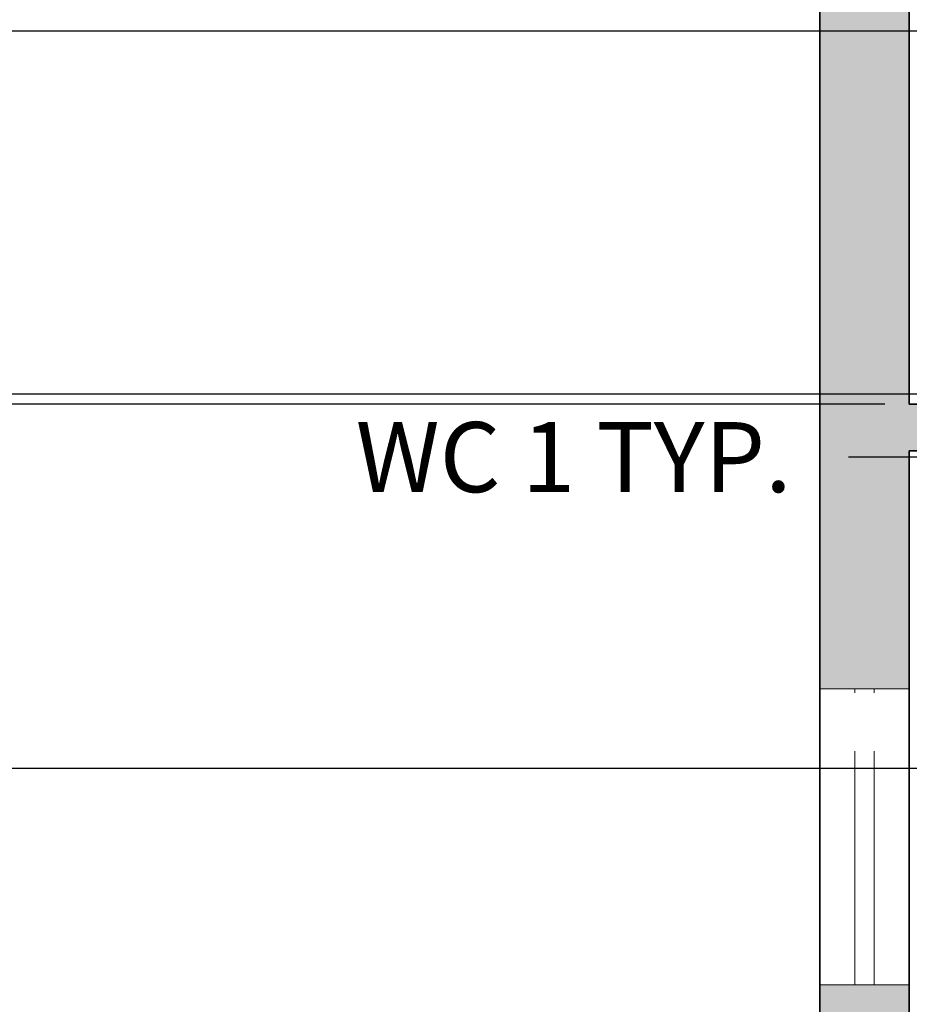
# Model space of a CAD drawing. Units: metres. Extents: x 4298.5 to 4325.2, y 2075 to 2095.8.
# Tile 12 of 35: x 4303.6 to 4305.9, y 2080.5 to 2083. Entities that reach past the tile are written whole.
import ezdxf

# ---------------------------------------------------------------- set-up
doc = ezdxf.new("R2010")
doc.units = ezdxf.units.M
doc.linetypes.add('ACAD_ISO02W100', pattern=[15, 12, -3])
for name, color, linetype, lineweight in [('A-ANNO-DIMS', 2, 'Continuous', 18), ('A-GLAZ', 4, 'Continuous', 18), ('A-GLAZ-OVHD', 4, 'ACAD_ISO02W100', 13), ('A-WALL', 7, 'Continuous', 35), ('A-WALL-PATT', 252, 'Continuous', 13)]:
    doc.layers.add(name, color=color, linetype=linetype, lineweight=lineweight)
doc.styles.get("Standard").update_dxf_attribs({"font": 'arial.ttf'})
doc.dimstyles.get("Standard").update_dxf_attribs({"dimtxt": 0.18, "dimasz": 0.18, "dimexe": 0.18, "dimexo": 0.0625, "dimgap": 0.09, "dimtad": 0, "dimtih": 1, "dimtoh": 1, "dimdec": 4, "dimzin": 0, "dimdsep": 46, "dimtxsty": 'Standard', "dimcen": 0.09, "dimadec": 0, "dimazin": 0, "dimtfac": 1, "dimtdec": 4, "dimtofl": 0, "dimtmove": 0, "dimatfit": 3, "dimfxl": 1, "dimtolj": 1, "dimtzin": 0, "dimarcsym": 0})

# ---------------------------------------------------------------- blocks, each defined once
blk = doc.blocks.new('WIN-760-GLASS-HIGH')
at = {"ltscale": 0.05}
for p, q in [((0, 0.76), (0, 0)), ((0.05, 0.76), (0.05, 0))]:
    blk.add_line(p, q, dxfattribs=at)
blk = doc.blocks.new('*D31')
at = {"layer": 'A-ANNO-DIMS', "color": 0, "lineweight": -2, "transparency": 16777216}
for p, q in [((4305.9147, 2081.8585), (4305.9147, 2082.1019)), ((4306.7541, 2081.8585), (4306.7541, 2082.1019)), ((4305.9147, 2081.9219), (4305.7347, 2081.9219)), ((4306.5741, 2081.9219), (4306.0947, 2081.9219))]:
    blk.add_line(p, q, dxfattribs=at)
at = {"layer": 'A-ANNO-DIMS', "color": 0, "transparency": 16777216}
for points in [[(4306.0947, 2081.9519), (4306.0947, 2081.8919), (4305.9147, 2081.9219)], [(4306.5741, 2081.9519), (4306.5741, 2081.8919), (4306.7541, 2081.9219)]]:
    blk.add_solid(points, dxfattribs=at)
at = {"layer": 'Defpoints', "color": 0, "transparency": 16777216}
for p in [(4305.9147, 2081.9219), (4305.9147, 2081.796), (4306.7541, 2081.796)]:
    blk.add_point(p, dxfattribs=at)
at = {"layer": 'A-ANNO-DIMS', "color": 0, "transparency": 16777216, "insert": (4305.0285, 2081.9219), "char_height": 0.18, "attachment_point": 5}
blk.add_mtext('\\A1;WC 1 TYP.', dxfattribs=at)
blk = doc.blocks.new('*D47')
at = {"layer": 'A-ANNO-DIMS', "color": 0, "lineweight": -2, "transparency": 16777216}
for p, q in [((4300.4306, 2084.4956), (4300.4306, 2074.9896)), ((4322.8106, 2084.4956), (4322.8106, 2074.9896)), ((4300.6106, 2075.1696), (4311.2252, 2075.1696)), ((4322.6306, 2075.1696), (4312.016, 2075.1696))]:
    blk.add_line(p, q, dxfattribs=at)
at = {"layer": 'A-ANNO-DIMS', "color": 0, "transparency": 16777216}
for points in [[(4300.6106, 2075.1996), (4300.6106, 2075.1396), (4300.4306, 2075.1696)], [(4322.6306, 2075.1996), (4322.6306, 2075.1396), (4322.8106, 2075.1696)]]:
    blk.add_solid(points, dxfattribs=at)
at = {"layer": 'Defpoints', "color": 0, "transparency": 16777216}
for p in [(4300.4306, 2084.5581), (4322.8106, 2084.5581), (4322.8106, 2075.1696)]:
    blk.add_point(p, dxfattribs=at)
at = {"layer": 'A-ANNO-DIMS', "color": 0, "transparency": 16777216, "insert": (4311.6206, 2075.1696), "char_height": 0.18, "attachment_point": 5}
blk.add_mtext('\\A1;22.38', dxfattribs=at)
blk = doc.blocks.new('*D51')
at = {"layer": 'A-ANNO-DIMS', "color": 0, "lineweight": -2, "transparency": 16777216}
for p, q in [((4305.5981, 2084.5581), (4299.0921, 2084.5581)), ((4299.2721, 2084.3781), (4299.2721, 2082.375)), ((4299.2721, 2080.0081), (4299.2721, 2082.0111)), ((4305.5981, 2079.8281), (4299.0921, 2079.8281))]:
    blk.add_line(p, q, dxfattribs=at)
at = {"layer": 'A-ANNO-DIMS', "color": 0, "transparency": 16777216}
for points in [[(4299.2421, 2084.3781), (4299.3021, 2084.3781), (4299.2721, 2084.5581)], [(4299.2421, 2080.0081), (4299.3021, 2080.0081), (4299.2721, 2079.8281)]]:
    blk.add_solid(points, dxfattribs=at)
at = {"layer": 'Defpoints', "color": 0, "transparency": 16777216}
for p in [(4305.6606, 2084.5581), (4299.2721, 2079.8281), (4305.6606, 2079.8281)]:
    blk.add_point(p, dxfattribs=at)
at = {"layer": 'A-ANNO-DIMS', "color": 0, "transparency": 16777216, "insert": (4299.2721, 2082.1931), "char_height": 0.18, "attachment_point": 5}
blk.add_mtext('\\A1;4.73', dxfattribs=at)
blk = doc.blocks.new('*D56')
at = {"layer": 'A-ANNO-DIMS', "color": 0, "lineweight": -2, "transparency": 16777216}
for p, q in [((4305.8281, 2085.0581), (4299.0921, 2085.0581)), ((4299.2721, 2084.8781), (4299.2721, 2083.74)), ((4299.2721, 2082.2381), (4299.2721, 2083.3761)), ((4305.8281, 2082.0581), (4299.0921, 2082.0581))]:
    blk.add_line(p, q, dxfattribs=at)
at = {"layer": 'A-ANNO-DIMS', "color": 0, "transparency": 16777216}
for points in [[(4299.2421, 2084.8781), (4299.3021, 2084.8781), (4299.2721, 2085.0581)], [(4299.2421, 2082.2381), (4299.3021, 2082.2381), (4299.2721, 2082.0581)]]:
    blk.add_solid(points, dxfattribs=at)
at = {"layer": 'Defpoints', "color": 0, "transparency": 16777216}
for p in [(4299.2721, 2085.0581), (4305.8906, 2085.0581), (4305.8906, 2082.0581)]:
    blk.add_point(p, dxfattribs=at)
at = {"layer": 'A-ANNO-DIMS', "color": 0, "transparency": 16777216, "insert": (4299.2721, 2083.5581), "char_height": 0.18, "attachment_point": 5}
blk.add_mtext('\\A1;3', dxfattribs=at)
blk = doc.blocks.new('*D62')
at = {"layer": 'A-ANNO-DIMS', "color": 0, "lineweight": -2, "transparency": 16777216}
for p, q in [((4312.1097, 2083.0153), (4299.0921, 2083.0153)), ((4299.2721, 2082.8353), (4299.2721, 2082.7313)), ((4299.2721, 2082.2635), (4299.2721, 2082.3674)), ((4312.1097, 2082.0835), (4299.0921, 2082.0835))]:
    blk.add_line(p, q, dxfattribs=at)
at = {"layer": 'A-ANNO-DIMS', "color": 0, "transparency": 16777216}
for points in [[(4299.2421, 2082.8353), (4299.3021, 2082.8353), (4299.2721, 2083.0153)], [(4299.2421, 2082.2635), (4299.3021, 2082.2635), (4299.2721, 2082.0835)]]:
    blk.add_solid(points, dxfattribs=at)
at = {"layer": 'Defpoints', "color": 0, "transparency": 16777216}
for p in [(4312.1722, 2083.0153), (4299.2721, 2082.0835), (4312.1722, 2082.0835)]:
    blk.add_point(p, dxfattribs=at)
at = {"layer": 'A-ANNO-DIMS', "color": 0, "transparency": 16777216, "insert": (4299.2721, 2082.5494), "char_height": 0.18, "attachment_point": 5}
blk.add_mtext('\\A1;0.93', dxfattribs=at)
blk = doc.blocks.new('*D63')
at = {"layer": 'A-ANNO-DIMS', "color": 0, "lineweight": -2, "transparency": 16777216}
for p, q in [((4312.1097, 2082.0835), (4299.0921, 2082.0835)), ((4299.2721, 2081.9035), (4299.2721, 2081.7847)), ((4299.2721, 2081.3021), (4299.2721, 2081.4209)), ((4312.1097, 2081.1221), (4299.0921, 2081.1221))]:
    blk.add_line(p, q, dxfattribs=at)
at = {"layer": 'A-ANNO-DIMS', "color": 0, "transparency": 16777216}
for points in [[(4299.2421, 2081.9035), (4299.3021, 2081.9035), (4299.2721, 2082.0835)], [(4299.2421, 2081.3021), (4299.3021, 2081.3021), (4299.2721, 2081.1221)]]:
    blk.add_solid(points, dxfattribs=at)
at = {"layer": 'Defpoints', "color": 0, "transparency": 16777216}
for p in [(4312.1722, 2082.0835), (4299.2721, 2081.1221), (4312.1722, 2081.1221)]:
    blk.add_point(p, dxfattribs=at)
at = {"layer": 'A-ANNO-DIMS', "color": 0, "transparency": 16777216, "insert": (4299.2721, 2081.6028), "char_height": 0.18, "attachment_point": 5}
blk.add_mtext('\\A1;0.96', dxfattribs=at)
blk = doc.blocks.new('*D64')
at = {"layer": 'A-ANNO-DIMS', "color": 0, "lineweight": -2, "transparency": 16777216}
for p, q in [((4312.1097, 2081.1221), (4299.0921, 2081.1221)), ((4299.2721, 2080.9421), (4299.2721, 2080.427)), ((4312.1097, 2080.247), (4299.0921, 2080.247)), ((4299.2721, 2080.247), (4299.2721, 2080.067)), ((4299.2721, 2080.067), (4299.0921, 2080.067))]:
    blk.add_line(p, q, dxfattribs=at)
at = {"layer": 'A-ANNO-DIMS', "color": 0, "transparency": 16777216}
for points in [[(4299.2421, 2080.9421), (4299.3021, 2080.9421), (4299.2721, 2081.1221)], [(4299.2421, 2080.427), (4299.3021, 2080.427), (4299.2721, 2080.247)]]:
    blk.add_solid(points, dxfattribs=at)
at = {"layer": 'Defpoints', "color": 0, "transparency": 16777216}
for p in [(4312.1722, 2081.1221), (4299.2721, 2080.247), (4312.1722, 2080.247)]:
    blk.add_point(p, dxfattribs=at)
at = {"layer": 'A-ANNO-DIMS', "color": 0, "transparency": 16777216, "insert": (4298.7681, 2080.067), "char_height": 0.18, "attachment_point": 5}
blk.add_mtext('\\A1;0.88', dxfattribs=at)

msp = doc.modelspace()

# ---------------------------------------------------------------- hatches: boundary and pattern name
at = {"layer": 'A-WALL-PATT'}
h = msp.add_hatch(color=256, dxfattribs=at)
h.dxf.hatch_style = 1
h.paths.add_polyline_path([(4308.7606, 2094.4781), (4308.1606, 2094.4781), (4307.4606, 2094.4781), (4307.4606, 2094.2481), (4308.2706, 2094.2481), (4308.2706, 2094.1281), (4308.3906, 2094.1281), (4308.3906, 2094.2481), (4308.7606, 2094.2481)])
h.paths.add_polyline_path([(4310.1206, 2094.4781), (4309.5206, 2094.4781), (4309.5206, 2094.2481), (4309.8906, 2094.2481), (4309.8906, 2092.2481), (4308.3906, 2092.2481), (4308.3906, 2093.4281), (4308.2706, 2093.4281), (4308.2706, 2092.0181), (4309.8906, 2092.0181), (4309.8906, 2087.0181), (4309.7706, 2087.0181), (4309.7706, 2086.7881), (4309.8906, 2086.7881), (4311.9406, 2086.7881), (4311.9406, 2087.0181), (4310.1206, 2087.0181), (4310.1206, 2089.0181), (4310.2406, 2089.0181), (4310.2406, 2089.1381), (4310.1206, 2089.1381), (4310.1206, 2092.0181), (4310.3078, 2092.0181), (4310.3078, 2092.2481), (4310.1206, 2092.2481)])
h.paths.add_polyline_path([(4311.7406, 2092.2481), (4311.0678, 2092.2481), (4311.0678, 2092.0181), (4311.7406, 2092.0181)], flags=17)
h.paths.add_polyline_path([(4313.1733, 2092.2481), (4312.5006, 2092.2481), (4312.5006, 2092.0181), (4313.1733, 2092.0181)])
h.paths.add_polyline_path([(4314.5378, 2092.2481), (4314.1206, 2092.2481), (4313.9333, 2092.2481), (4313.9333, 2092.0181), (4314.1206, 2092.0181), (4314.1206, 2087.0181), (4314.0006, 2087.0181), (4314.0006, 2086.7881), (4314.1206, 2086.7881), (4315.5718, 2086.7881), (4315.5718, 2087.0181), (4314.3506, 2087.0181), (4314.3506, 2092.0181), (4314.5378, 2092.0181)])
h.paths.add_polyline_path([(4315.9706, 2092.2481), (4315.2978, 2092.2481), (4315.2978, 2092.0181), (4315.9706, 2092.0181)])
h.paths.add_polyline_path([(4317.4033, 2092.2481), (4316.7306, 2092.2481), (4316.7306, 2092.0181), (4317.4033, 2092.0181)])
h.paths.add_polyline_path([(4318.9506, 2092.2481), (4318.3506, 2092.2481), (4318.1633, 2092.2481), (4318.1633, 2092.0181), (4318.3506, 2092.0181), (4318.3506, 2091.8981), (4318.5806, 2091.8981), (4318.5806, 2092.0181), (4318.9506, 2092.0181)])
h.paths.add_polyline_path([(4321.0106, 2092.2481), (4319.7106, 2092.2481), (4319.7106, 2092.0181), (4320.0806, 2092.0181), (4320.0806, 2090.0181), (4318.5806, 2090.0181), (4318.5806, 2091.1981), (4318.3506, 2091.1981), (4318.3506, 2090.0181), (4318.3506, 2087.0181), (4318.2306, 2087.0181), (4318.2306, 2086.7881), (4318.3506, 2086.7881), (4318.3506, 2086.3081), (4318.5806, 2086.3081), (4318.5806, 2089.7881), (4321.7806, 2089.7881), (4321.7806, 2090.0181), (4320.2006, 2090.0181), (4320.2006, 2092.0181), (4321.0106, 2092.0181)])
h.paths.add_polyline_path([(4322.8106, 2092.2481), (4321.7706, 2092.2481), (4321.7706, 2092.0181), (4322.5806, 2092.0181), (4322.5806, 2091.2831), (4322.8106, 2091.2831)])
h.paths.add_polyline_path([(4322.8106, 2090.5231), (4322.5806, 2090.5231), (4322.5806, 2089.7881), (4322.5806, 2089.5254), (4322.8106, 2089.5254), (4322.8106, 2090.0181)])
h.paths.add_polyline_path([(4322.8106, 2088.7654), (4322.5806, 2088.7654), (4322.5806, 2087.6681), (4322.8106, 2087.6681)])
h.paths.add_polyline_path([(4322.8106, 2086.9081), (4322.5806, 2086.9081), (4322.5806, 2085.8107), (4322.8106, 2085.8107)])
h.paths.add_polyline_path([(4322.8106, 2085.0507), (4322.5806, 2085.0507), (4322.5806, 2084.7881), (4318.5806, 2084.7881), (4318.5806, 2085.0581), (4318.5806, 2085.4081), (4318.3506, 2085.4081), (4318.3506, 2084.5581), (4318.3506, 2080.8581), (4318.4706, 2080.8581), (4318.4706, 2082.3281), (4319.2606, 2082.3281), (4319.2606, 2082.5581), (4318.5806, 2082.5581), (4318.5806, 2084.5581), (4320.0806, 2084.5581), (4320.0806, 2083.9381), (4320.3106, 2083.9381), (4320.3106, 2084.5581), (4322.8106, 2084.5581)])
h.paths.add_polyline_path([(4320.3106, 2083.1781), (4320.0806, 2083.1781), (4320.0806, 2082.5581), (4319.9606, 2082.5581), (4319.9606, 2082.3281), (4320.0806, 2082.3281), (4320.0806, 2081.5731), (4320.3106, 2081.5731)], flags=17)
h.paths.add_polyline_path([(4320.3106, 2080.8131), (4320.0806, 2080.8131), (4320.0806, 2080.0581), (4318.4286, 2080.0581), (4318.4286, 2079.8281), (4320.3106, 2079.8281)])
h.paths.add_polyline_path([(4317.3506, 2085.2881), (4316.5718, 2085.2881), (4316.5718, 2085.0581), (4317.3506, 2085.0581)])
h.paths.add_polyline_path([(4315.5718, 2085.2881), (4314.8434, 2085.2881), (4314.8434, 2085.0581), (4315.5718, 2085.0581)])
h.paths.add_polyline_path([(4313.8434, 2085.2881), (4312.9406, 2085.2881), (4312.9406, 2085.0581), (4313.8434, 2085.0581)])
h.paths.add_polyline_path([(4311.9406, 2085.2881), (4311.4406, 2085.2881), (4311.4406, 2085.0581), (4311.9406, 2085.0581)])
h.paths.add_polyline_path([(4317.3306, 2087.0181), (4316.5718, 2087.0181), (4316.5718, 2086.7881), (4317.3306, 2086.7881)])
h.paths.add_polyline_path([(4313.1006, 2089.1381), (4311.1406, 2089.1381), (4311.1406, 2089.0181), (4312.9806, 2089.0181), (4312.9806, 2087.0181), (4312.9406, 2087.0181), (4312.9406, 2086.7881), (4313.1006, 2086.7881), (4313.1006, 2087.0181)])
h.paths.add_polyline_path([(4307.5515, 2087.0181), (4305.8906, 2087.0181), (4305.8906, 2092.2481), (4305.8906, 2094.2481), (4306.7006, 2094.2481), (4306.7006, 2094.4781), (4305.6606, 2094.4781), (4305.6606, 2092.2481), (4305.2906, 2092.2481), (4305.2906, 2092.0181), (4305.6606, 2092.0181), (4305.6606, 2090.0181), (4304.1606, 2090.0181), (4304.1606, 2091.1981), (4304.0406, 2091.1981), (4304.0406, 2089.9081), (4301.5606, 2089.9081), (4301.5606, 2089.7881), (4304.0406, 2089.7881), (4305.6606, 2089.7881), (4305.6606, 2086.6381), (4305.8906, 2086.6381), (4305.8906, 2086.7881), (4307.5515, 2086.7881)])
h.paths.add_polyline_path([(4307.5515, 2085.2881), (4305.8906, 2085.2881), (4305.8906, 2085.4381), (4305.6606, 2085.4381), (4305.6606, 2084.7881), (4305.2906, 2084.7881), (4305.2906, 2084.5581), (4305.6606, 2084.5581), (4305.6606, 2084.02), (4305.8906, 2084.02), (4305.8906, 2084.5581), (4305.8906, 2085.0581), (4307.5515, 2085.0581)])
h.paths.add_polyline_path([(4310.2406, 2085.2881), (4308.5515, 2085.2881), (4308.5515, 2085.0581), (4310.2406, 2085.0581)])
h.paths.add_polyline_path([(4317.4286, 2080.0581), (4316.5718, 2080.0581), (4316.5718, 2079.8281), (4317.4286, 2079.8281)])
h.paths.add_polyline_path([(4315.5718, 2080.0581), (4314.8434, 2080.0581), (4314.8434, 2079.8281), (4315.5718, 2079.8281)])
h.paths.add_polyline_path([(4313.8434, 2080.0581), (4312.9406, 2080.0581), (4312.9406, 2079.8281), (4313.8434, 2079.8281)])
h.paths.add_polyline_path([(4311.9406, 2080.0581), (4311.4406, 2080.0581), (4311.4406, 2079.8281), (4311.9406, 2079.8281)])
h.paths.add_polyline_path([(4310.2406, 2080.0581), (4310.1206, 2080.0581), (4310.1206, 2084.0381), (4309.8906, 2084.0381), (4309.8906, 2080.0581), (4309.1606, 2080.0581), (4309.1606, 2079.8281), (4310.2406, 2079.8281)])
h.paths.add_polyline_path([(4308.1606, 2080.0581), (4307.5106, 2080.0581), (4307.5106, 2080.1781), (4307.3906, 2080.1781), (4307.3906, 2080.0581), (4305.8906, 2080.0581), (4305.8906, 2080.567), (4305.6606, 2080.567), (4305.6606, 2079.8281), (4308.1606, 2079.8281)])
h.paths.add_polyline_path([(4307.5106, 2081.9381), (4309.0906, 2081.9381), (4309.0906, 2082.0581), (4305.8906, 2082.0581), (4305.8906, 2083.26), (4305.6606, 2083.26), (4305.6606, 2081.327), (4305.8906, 2081.327), (4305.8906, 2081.9381), (4307.3906, 2081.9381), (4307.3906, 2080.8781), (4307.5106, 2080.8781)])
h.paths.add_polyline_path([(4304.5306, 2084.7881), (4302.7306, 2084.7881), (4302.7306, 2084.5581), (4304.5306, 2084.5581)])
h.paths.add_polyline_path([(4301.9706, 2084.7881), (4300.6606, 2084.7881), (4300.6606, 2085.0249), (4300.4306, 2085.0249), (4300.4306, 2084.5581), (4301.9706, 2084.5581)])
h.paths.add_polyline_path([(4300.6606, 2086.8843), (4300.4306, 2086.8843), (4300.4306, 2085.7849), (4300.6606, 2085.7849)])
h.paths.add_polyline_path([(4300.6606, 2089.1618), (4300.4306, 2089.1618), (4300.4306, 2087.6443), (4300.6606, 2087.6443)])
h.paths.add_polyline_path([(4300.6606, 2091.0212), (4300.4306, 2091.0212), (4300.4306, 2089.9218), (4300.6606, 2089.9218)])
h.paths.add_polyline_path([(4300.6606, 2092.0181), (4301.9706, 2092.0181), (4301.9706, 2092.2481), (4300.4306, 2092.2481), (4300.4306, 2091.7812), (4300.6606, 2091.7812)])
h.paths.add_polyline_path([(4304.5306, 2092.2481), (4302.7306, 2092.2481), (4302.7306, 2092.0181), (4304.0406, 2092.0181), (4304.0406, 2091.8981), (4304.1606, 2091.8981), (4304.1606, 2092.0181), (4304.5306, 2092.0181)], flags=17)

# ---------------------------------------------------------------- linework, layer by layer
at = {"layer": 'A-GLAZ'}
for p, q in [((4305.6606, 2081.327), (4305.8906, 2081.327)), ((4305.6606, 2080.567), (4305.8906, 2080.567))]:
    msp.add_line(p, q, dxfattribs=at)
at = {"layer": 'A-WALL'}
for p, q in [((4305.6606, 2084.5581), (4305.6606, 2079.8281)), ((4305.8906, 2084.5581), (4305.8906, 2082.0581)), ((4305.8906, 2082.0581), (4309.0906, 2082.0581)), ((4305.8906, 2081.9381), (4307.3906, 2081.9381)), ((4305.8906, 2081.9381), (4305.8906, 2080.0581))]:
    msp.add_line(p, q, dxfattribs=at)

# ---------------------------------------------------------------- block references
at = {"layer": 'A-GLAZ-OVHD', "rotation": 180}
msp.add_blockref('WIN-760-GLASS-HIGH', (4305.8006, 2081.327), dxfattribs=at)

# ---------------------------------------------------------------- dimensions: what is measured, and where the dimension line sits
at = {"layer": 'A-ANNO-DIMS'}
for base, p1, p2, override, picture, middle in [((4299.2721, 2085.0581), (4305.8906, 2082.0581), (4305.8906, 2085.0581), {"dimdec": 0, "dimlfac": 1, "dimrnd": 0, "dimzin": 0, "dimdsep": 46, "dimlunit": 2}, '*D56', (4299.2721, 2083.5581)), ((4299.2721, 2079.8281), (4305.6606, 2084.5581), (4305.6606, 2079.8281), {"dimdec": 2, "dimlfac": 1, "dimrnd": 0, "dimzin": 0, "dimdsep": 46, "dimlunit": 2}, '*D51', (4299.2721, 2082.1931)), ((4299.2721, 2082.0835), (4312.1722, 2083.0153), (4312.1722, 2082.0835), {"dimdec": 2, "dimlfac": 1, "dimrnd": 0, "dimzin": 0, "dimdsep": 46, "dimlunit": 2}, '*D62', (4299.2721, 2082.5494)), ((4299.2721, 2081.1221), (4312.1722, 2082.0835), (4312.1722, 2081.1221), {"dimdec": 2, "dimlfac": 1, "dimrnd": 0, "dimzin": 0, "dimdsep": 46, "dimlunit": 2}, '*D63', (4299.2721, 2081.6028)), ((4299.2721, 2080.247), (4312.1722, 2081.1221), (4312.1722, 2080.247), {"dimdec": 2, "dimlfac": 1, "dimrnd": 0, "dimzin": 0, "dimdsep": 46, "dimlunit": 2}, '*D64', (4298.7681, 2080.067))]:
    dim = msp.add_linear_dim(base=base, p1=p1, p2=p2, angle=90, dimstyle='Standard', override=override, dxfattribs=at)
    dim.commit()
    dim.dimension.update_dxf_attribs({"geometry": picture, "text_midpoint": middle})
dim = msp.add_linear_dim(base=(4322.8106, 2075.1696), p1=(4300.4306, 2084.5581), p2=(4322.8106, 2084.5581), dimstyle='Standard', override={"dimdec": 2, "dimlfac": 1, "dimrnd": 0, "dimzin": 0, "dimdsep": 46, "dimlunit": 2}, dxfattribs=at)
dim.commit()
dim.dimension.update_dxf_attribs({"geometry": '*D47', "text_midpoint": (4311.6206, 2075.1696)})
dim = msp.add_linear_dim(base=(4305.9147, 2081.9219), p1=(4306.7541, 2081.796), p2=(4305.9147, 2081.796), angle=180, text='WC <> TYP.', dimstyle='Standard', override={"dimdec": 0, "dimlfac": 1, "dimrnd": 0, "dimzin": 0, "dimdsep": 46, "dimlunit": 2}, dxfattribs=at)
dim.commit()
dim.dimension.update_dxf_attribs({"geometry": '*D31', "text_midpoint": (4305.0285, 2081.9219)})

doc.saveas('drawing.dxf')
